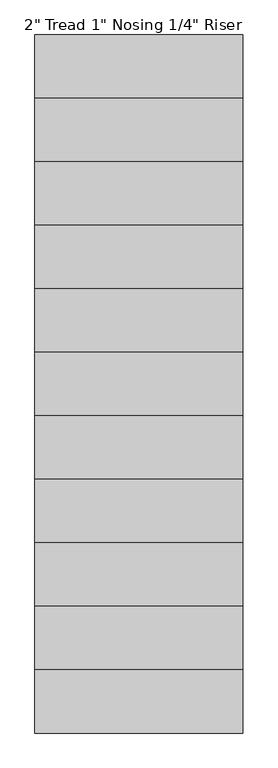
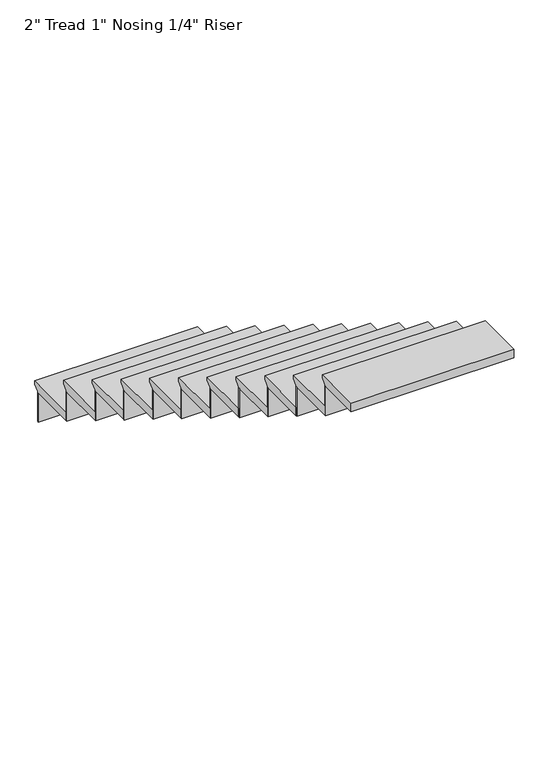
"""IFC4 building model written with IfcOpenShell, lengths in millimetres: stair flight geometry."""

from ifc_helpers import new_model, si_unit, frame, origin, place, context, project, spatial, polyline, outline, extrude, source, transform, mapped, element, save


def stair_flight_ca9b9272(model_context):
    return source(origin(), model_context, "Body", "SweptSolid", [
        extrude(outline(polyline([(520.7660813, 1905.0), (825.5660813, 1905.0), (825.5660813, 1885.95), (800.1660813, 1860.55), (800.1660813, 1854.2), (520.7660813, 1854.2), (520.7660813, 1905.0)])), frame((8683.6260838, 0.0, 0.0), z_axis=(1.0, 0.0, 0.0), x_axis=(0.0, 1.0, 0.0)), (0.0, 0.0, 1.0), 914.4),
        extrude(outline(polyline([(8683.6260838, 793.8160813), (8683.6260838, 800.1660813), (9598.0260838, 800.1660813), (9598.0260838, 793.8160813), (8683.6260838, 793.8160813)])), frame((0.0, 0.0, 1681.0181818), z_axis=(0.0, 0.0, 1.0), x_axis=(1.0, 0.0, 0.0)), (0.0, 0.0, 1.0), 173.1818182),
        extrude(outline(polyline([(8683.6260838, 514.4160813), (8683.6260838, 520.7660813), (9598.0260838, 520.7660813), (9598.0260838, 514.4160813), (8683.6260838, 514.4160813)])), frame((0.0, 0.0, 1854.2), z_axis=(0.0, 0.0, 1.0), x_axis=(1.0, 0.0, 0.0)), (0.0, 0.0, 1.0), 173.1818182),
        extrude(outline(polyline([(241.3660813, 2078.1818182), (546.1660813, 2078.1818182), (546.1660813, 2059.1318182), (520.7660813, 2033.7318182), (520.7660813, 2027.3818182), (241.3660813, 2027.3818182), (241.3660813, 2078.1818182)])), frame((8683.6260838, 0.0, 0.0), z_axis=(1.0, 0.0, 0.0), x_axis=(0.0, 1.0, 0.0)), (0.0, 0.0, 1.0), 914.4),
        extrude(outline(polyline([(8683.6260838, 235.0160813), (8683.6260838, 241.3660813), (9598.0260838, 241.3660813), (9598.0260838, 235.0160813), (8683.6260838, 235.0160813)])), frame((0.0, 0.0, 2027.3818182), z_axis=(0.0, 0.0, 1.0), x_axis=(1.0, 0.0, 0.0)), (0.0, 0.0, 1.0), 173.1818182),
        extrude(outline(polyline([(-38.0339187, 2251.3636364), (266.7660813, 2251.3636364), (266.7660813, 2232.3136364), (241.3660813, 2206.9136364), (241.3660813, 2200.5636364), (-38.0339187, 2200.5636364), (-38.0339187, 2251.3636364)])), frame((8683.6260838, 0.0, 0.0), z_axis=(1.0, 0.0, 0.0), x_axis=(0.0, 1.0, 0.0)), (0.0, 0.0, 1.0), 914.4),
        extrude(outline(polyline([(8683.6260838, -44.3839187), (8683.6260838, -38.0339187), (9598.0260838, -38.0339187), (9598.0260838, -44.3839187), (8683.6260838, -44.3839187)])), frame((0.0, 0.0, 2200.5636364), z_axis=(0.0, 0.0, 1.0), x_axis=(1.0, 0.0, 0.0)), (0.0, 0.0, 1.0), 173.1818182),
        extrude(outline(polyline([(-317.4339187, 2424.5454545), (-12.6339187, 2424.5454545), (-12.6339187, 2405.4954545), (-38.0339187, 2380.0954545), (-38.0339187, 2373.7454545), (-317.4339187, 2373.7454545), (-317.4339187, 2424.5454545)])), frame((8683.6260838, 0.0, 0.0), z_axis=(1.0, 0.0, 0.0), x_axis=(0.0, 1.0, 0.0)), (0.0, 0.0, 1.0), 914.4),
        extrude(outline(polyline([(8683.6260838, -323.7839187), (8683.6260838, -317.4339187), (9598.0260838, -317.4339187), (9598.0260838, -323.7839187), (8683.6260838, -323.7839187)])), frame((0.0, 0.0, 2373.7454545), z_axis=(0.0, 0.0, 1.0), x_axis=(1.0, 0.0, 0.0)), (0.0, 0.0, 1.0), 173.1818182),
        extrude(outline(polyline([(-596.8339187, 2597.7272727), (-292.0339187, 2597.7272727), (-292.0339187, 2578.6772727), (-317.4339187, 2553.2772727), (-317.4339187, 2546.9272727), (-596.8339187, 2546.9272727), (-596.8339187, 2597.7272727)])), frame((8683.6260838, 0.0, 0.0), z_axis=(1.0, 0.0, 0.0), x_axis=(0.0, 1.0, 0.0)), (0.0, 0.0, 1.0), 914.4),
        extrude(outline(polyline([(8683.6260838, -603.1839187), (8683.6260838, -596.8339187), (9598.0260838, -596.8339187), (9598.0260838, -603.1839187), (8683.6260838, -603.1839187)])), frame((0.0, 0.0, 2546.9272727), z_axis=(0.0, 0.0, 1.0), x_axis=(1.0, 0.0, 0.0)), (0.0, 0.0, 1.0), 173.1818182),
        extrude(outline(polyline([(-876.2339187, 2770.9090909), (-571.4339187, 2770.9090909), (-571.4339187, 2751.8590909), (-596.8339187, 2726.4590909), (-596.8339187, 2720.1090909), (-876.2339187, 2720.1090909), (-876.2339187, 2770.9090909)])), frame((8683.6260838, 0.0, 0.0), z_axis=(1.0, 0.0, 0.0), x_axis=(0.0, 1.0, 0.0)), (0.0, 0.0, 1.0), 914.4),
        extrude(outline(polyline([(8683.6260838, -882.5839187), (8683.6260838, -876.2339187), (9598.0260838, -876.2339187), (9598.0260838, -882.5839187), (8683.6260838, -882.5839187)])), frame((0.0, 0.0, 2720.1090909), z_axis=(0.0, 0.0, 1.0), x_axis=(1.0, 0.0, 0.0)), (0.0, 0.0, 1.0), 173.1818182),
        extrude(outline(polyline([(-1155.6339187, 2944.0909091), (-850.8339187, 2944.0909091), (-850.8339187, 2925.0409091), (-876.2339187, 2899.6409091), (-876.2339187, 2893.2909091), (-1155.6339187, 2893.2909091), (-1155.6339187, 2944.0909091)])), frame((8683.6260838, 0.0, 0.0), z_axis=(1.0, 0.0, 0.0), x_axis=(0.0, 1.0, 0.0)), (0.0, 0.0, 1.0), 914.4),
        extrude(outline(polyline([(8683.6260838, -1161.9839187), (8683.6260838, -1155.6339187), (9598.0260838, -1155.6339187), (9598.0260838, -1161.9839187), (8683.6260838, -1161.9839187)])), frame((0.0, 0.0, 2893.2909091), z_axis=(0.0, 0.0, 1.0), x_axis=(1.0, 0.0, 0.0)), (0.0, 0.0, 1.0), 173.1818182),
        extrude(outline(polyline([(-1435.0339187, 3117.2727273), (-1130.2339187, 3117.2727273), (-1130.2339187, 3098.2227273), (-1155.6339187, 3072.8227273), (-1155.6339187, 3066.4727273), (-1435.0339187, 3066.4727273), (-1435.0339187, 3117.2727273)])), frame((8683.6260838, 0.0, 0.0), z_axis=(1.0, 0.0, 0.0), x_axis=(0.0, 1.0, 0.0)), (0.0, 0.0, 1.0), 914.4),
        extrude(outline(polyline([(8683.6260838, -1441.3839187), (8683.6260838, -1435.0339187), (9598.0260838, -1435.0339187), (9598.0260838, -1441.3839187), (8683.6260838, -1441.3839187)])), frame((0.0, 0.0, 3066.4727273), z_axis=(0.0, 0.0, 1.0), x_axis=(1.0, 0.0, 0.0)), (0.0, 0.0, 1.0), 173.1818182),
        extrude(outline(polyline([(-1714.4339187, 3290.4545455), (-1409.6339187, 3290.4545455), (-1409.6339187, 3271.4045455), (-1435.0339187, 3246.0045455), (-1435.0339187, 3239.6545455), (-1714.4339187, 3239.6545455), (-1714.4339187, 3290.4545455)])), frame((8683.6260838, 0.0, 0.0), z_axis=(1.0, 0.0, 0.0), x_axis=(0.0, 1.0, 0.0)), (0.0, 0.0, 1.0), 914.4),
        extrude(outline(polyline([(8683.6260838, -1720.7839187), (8683.6260838, -1714.4339187), (9598.0260838, -1714.4339187), (9598.0260838, -1720.7839187), (8683.6260838, -1720.7839187)])), frame((0.0, 0.0, 3239.6545455), z_axis=(0.0, 0.0, 1.0), x_axis=(1.0, 0.0, 0.0)), (0.0, 0.0, 1.0), 173.1818182),
        extrude(outline(polyline([(-1993.8339187, 3463.6363636), (-1689.0339187, 3463.6363636), (-1689.0339187, 3444.5863636), (-1714.4339187, 3419.1863636), (-1714.4339187, 3412.8363636), (-1993.8339187, 3412.8363636), (-1993.8339187, 3463.6363636)])), frame((8683.6260838, 0.0, 0.0), z_axis=(1.0, 0.0, 0.0), x_axis=(0.0, 1.0, 0.0)), (0.0, 0.0, 1.0), 914.4),
        extrude(outline(polyline([(8683.6260838, -2000.1839187), (8683.6260838, -1993.8339187), (9598.0260838, -1993.8339187), (9598.0260838, -2000.1839187), (8683.6260838, -2000.1839187)])), frame((0.0, 0.0, 3412.8363636), z_axis=(0.0, 0.0, 1.0), x_axis=(1.0, 0.0, 0.0)), (0.0, 0.0, 1.0), 173.1818182),
        extrude(outline(polyline([(-2247.8339187, 3636.8181818), (-1968.4339187, 3636.8181818), (-1968.4339187, 3617.7681818), (-1993.8339187, 3592.3681818), (-1993.8339187, 3586.0181818), (-2247.8339187, 3586.0181818), (-2247.8339187, 3636.8181818)])), frame((8683.6260838, 0.0, 0.0), z_axis=(1.0, 0.0, 0.0), x_axis=(0.0, 1.0, 0.0)), (0.0, 0.0, 1.0), 914.4),
    ])


if __name__ == "__main__":
    model = new_model("IFC4")
    model_context = context("Model", 3, world=origin())
    ifc_project = project(units=[si_unit("LENGTHUNIT", "METRE", prefix="MILLI")], contexts=[model_context])
    site = spatial("IfcSite", under=ifc_project)
    building = spatial("IfcBuilding", under=site)
    placement = place(None, origin())
    stair_flight_shape = stair_flight_ca9b9272(model_context)
    element("IfcStairFlight", 1, ObjectType="2\" Tread 1\" Nosing 1/4\" Riser", at=placement, inside=building, context=model_context, shape_type="MappedRepresentation", body=[
        mapped(stair_flight_shape, transform((0.0, 0.0, 0.0), x_axis=(1.0, 0.0, 0.0), y_axis=(0.0, 1.0, 0.0), z_axis=(0.0, 0.0, 1.0))),
    ])
    save(model, "model.ifc")
